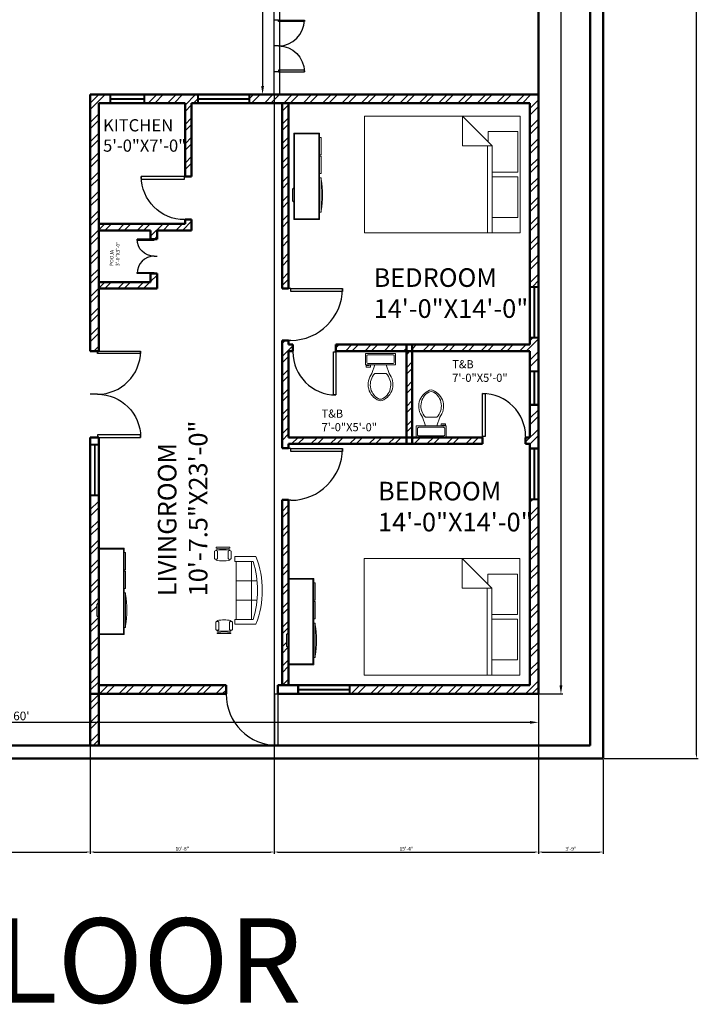
# Model space of a CAD drawing. Units: inches. Extents: x -12550 to 6516, y 1273 to 18700.
# Tile 17 of 19: x 6043 to 6516, y 1273 to 1958. Entities that reach past the tile are written whole.
import ezdxf

# ---------------------------------------------------------------- set-up
doc = ezdxf.new("R2010")
doc.units = ezdxf.units.IN
for name, color, linetype, lineweight in [('A-ANNO-DIMS', 2, 'Continuous', 18), ('A-ANNO-TEXT', 7, 'Continuous', 25), ('A-AREA-IDEN', 1, 'Continuous', 18), ('A-DOOR', 5, 'Continuous', 25), ('A-EQPM', 4, 'Continuous', 25), ('A-FURN', 8, 'Continuous', 18), ('A-GLAZ', 3, 'Continuous', 25), ('A-WALL', 7, 'Continuous', 50), ('A-WALL-PATT', 8, 'Continuous', 13)]:
    doc.layers.add(name, color=color, linetype=linetype, lineweight=lineweight)
doc.styles.get("Standard").update_dxf_attribs({"font": 'arial.ttf'})
doc.dimstyles.new('ISO-25', dxfattribs={"dimtxt": 2.5, "dimasz": 2.5, "dimexe": 1.25, "dimexo": 0.625, "dimtad": 1, "dimlunit": 4, "dimtxsty": 'Standard', "dimcen": 2.5, "dimadec": 0, "dimazin": 0, "dimtfac": 1, "dimtmove": 0, "dimatfit": 3, "dimfxl": 1, "dimarcsym": 0})
pattern_1 = [(45, (3666.851, 0), (-6.735192, 6.735192), []), (45, (3671.341, 0), (-6.735192, 6.735192), [])]

# ---------------------------------------------------------------- blocks, each defined once
blk = doc.blocks.new('*U2')
for p, q in [((0, 0), (0, -5)), ((30, 0), (30, -5))]:
    blk.add_line(p, q)
blk.add_lwpolyline([(0, 0), (0, 30), (1.75, 30), (1.75, 0)], close=True)
blk.add_arc((0, 0), 30, 0, 90)
blk = doc.blocks.new('Bed - Queen')
for p, q in [((0, -80.00003), (0, 0)), ((0, 0), (59.99999, 0)), ((59.99999, 0), (59.99999, -80.00003)), ((7.99999, -1.2), (28.79998, -1.2)), ((7.99999, -14.4), (7.99999, -1.2)), ((28.79998, -1.2), (28.79998, -14.4)), ((31.19999, -1.2), (51.99999, -1.2)), ((31.19999, -14.4), (31.19999, -1.2)), ((51.99999, -1.2), (51.99999, -16.4)), ((0, -14.4), (44.8, -14.4)), ((59.99999, -29.6), (44.8, -14.4)), ((44.8, -14.4), (44.8, -29.6)), ((44.8, -16.8), (0, -16.8)), ((51.99999, -16.4), (46.79936, -16.4)), ((44.8, -29.6), (59.99999, -29.6)), ((59.99999, -80.00003), (0, -80.00003))]:
    blk.add_line(p, q)
blk = doc.blocks.new('Toilet - top')
for p, q in [((9.5, -6), (9.5, -2)), ((-10, -8.5), (-8, -8.5)), ((-10, -9.5), (-10, -8.5)), ((-7, -9.5), (-10, -9.5)), ((-8, -8.5), (-8, -8)), ((-7, -8), (-7, -9.5)), ((-4, -8), (-6, -14)), ((4, -8), (6, -14)), ((4, -14), (-4, -14))]:
    blk.add_line(p, q)
blk.add_lwpolyline([(10.5, -8), (10.5, 0), (-10.5, 0), (-10.5, -8)], close=True)
for points in [[(-9.5, -2), (-9.5, -6)], [(8.5, -1), (-8.5, -1)], [(-8.5, -7), (8.5, -7)]]:
    blk.add_lwpolyline(points)
for centre, radius, start, end in [((-8.62, -1.88), 0.884, 81.8699, 188.1301), ((-8.62, -6.12), 0.884, 171.8699, 278.1301), ((8.62, -1.88), 0.884, 351.8699, 98.1301), ((8.62, -6.12), 0.884, 261.8699, 8.1301), ((3.52, -21.58), 12.17, 141.46911, 247.97143), ((4.2, -21.82), 11.33, 136.36773, 238.94682), ((-3.52, -21.58), 12.17, 292.02843, 38.53071), ((-4.2, -21.82), 11.33, 301.05301, 43.63209), ((0, -27.88), 4, 245.73182, 294.26817), ((0, -29), 4, 254.86053, 285.13947)]:
    blk.add_arc(centre, radius, start, end)
blk = doc.blocks.new('Entertainment Center')
for p, q in [((-4, 0), (-5, -1)), ((4, 0), (-4, 0)), ((5, -1), (4, 0)), ((-17, -19), (-17, -1)), ((-17, -1), (43, -1)), ((-16.5, -18.5), (-16.5, -1.5)), ((-16.5, -1.5), (42.5, -1.5)), ((42.5, -1.5), (42.5, -18.5)), ((43, -1), (43, -19)), ((43, -19), (-17, -19)), ((42.5, -18.5), (-16.5, -18.5)), ((-12, -20), (-12, -19)), ((12, -20), (-12, -20)), ((12, -19), (12, -20)), ((15, -20), (15, -19)), ((27, -20), (15, -20)), ((27, -19), (27, -20)), ((28, -20), (28, -19)), ((40, -20), (28, -20)), ((40, -19), (40, -20))]:
    blk.add_line(p, q)
blk.add_arc((0, 40), 61, 259.6111, 280.3889)
blk = doc.blocks.new('Sofa - Roundback 7 ft.')
for p, q in [((-36.000027, -34), (-36.000027, -11.4696)), ((-12.00002, -32.4421), (-12.00003, -6.5971)), ((11.99997, -32.4421), (11.99998, -6.5971)), ((35.99998, -34), (35.99998, -11.4696)), ((-35.999844, -13.3819), (35.9998, -13.3819)), ((-36.000027, -32.4421), (35.99998, -32.4421))]:
    blk.add_line(p, q)
for points in [[(-36.000027, -34), (-42.000027, -34), (-42.000027, -8)], [(41.99998, -8), (41.99998, -34), (35.99998, -34)]]:
    blk.add_lwpolyline(points)
for centre, radius, start, end in [((0, -114.25), 114.25, 68.43141, 111.5686), ((-0.00001, -127.1968), 121.1968, 72.72033, 107.2797)]:
    blk.add_arc(centre, radius, start, end)
blk = doc.blocks.new('Chair - Desk')
for p, q in [((-8.5, 0), (-8.5, -1)), ((-8.5, 0), (8.5, 0)), ((8.5, 0), (8.5, -1)), ((-10.5, -5), (-10.5, -14)), ((-8.5, -3), (-8.5, -4)), ((-8.5, -3), (8.5, -3)), ((-6.5, -14), (-6.5, -5)), ((-2, -3), (-2, -1.9355)), ((2, -1.9576), (2, -3)), ((6.5, -5), (6.5, -14)), ((8.5, -3), (8.5, -4)), ((10.5, -14), (10.5, -5)), ((-8.5, -15), (-8.5, -16)), ((8.5, -15), (8.5, -16))]:
    blk.add_line(p, q)
for centre, radius, start, end in [((-8.5, -6.5), 2.5, 36.8699, 143.1301), ((0, 34.625), 36.625, 256.5803, 283.4197), ((8.5, -6.5), 2.5, 36.8699, 143.1301), ((-8.5, -12.5), 2.5, 216.8699, 323.1301), ((0, 19.625), 36.625, 256.5803, 283.4197), ((8.5, -12.5), 2.5, 216.8699, 323.1301)]:
    blk.add_arc(centre, radius, start, end)
blk = doc.blocks.new('*D52')
at = {"layer": 'A-ANNO-DIMS', "color": 0, "lineweight": -2, "transparency": 16777216}
for p, q in [((6219.91, 2056.25), (6211.2, 2056.25)), ((6212.45, 2050.25), (6212.45, 1912.25)), ((6219.91, 1906.25), (6211.2, 1906.25))]:
    blk.add_line(p, q, dxfattribs=at)
at = {"layer": 'A-ANNO-DIMS', "color": 0, "transparency": 16777216}
for points in [[(6211.45, 2050.25), (6213.45, 2050.25), (6212.45, 2056.25)], [(6211.45, 1912.25), (6213.45, 1912.25), (6212.45, 1906.25)]]:
    blk.add_solid(points, dxfattribs=at)
at = {"layer": 'Defpoints', "color": 0, "transparency": 16777216}
for p in [(6220.54, 2056.25), (6212.45, 1906.25), (6220.54, 1906.25)]:
    blk.add_point(p, dxfattribs=at)
at = {"layer": 'A-ANNO-DIMS', "color": 0, "transparency": 16777216, "insert": (6208.76, 1981.25), "char_height": 6, "attachment_point": 5, "rotation": 90}
blk.add_mtext('12\'-6"', dxfattribs=at)
blk = doc.blocks.new('*D54')
at = {"layer": 'A-ANNO-DIMS', "color": 0, "lineweight": -2, "transparency": 16777216}
for p, q in [((6405.16, 2473.25), (6421.41, 2473.25)), ((6420.16, 2467.25), (6420.16, 1495.25)), ((6405.16, 1489.25), (6421.41, 1489.25))]:
    blk.add_line(p, q, dxfattribs=at)
at = {"layer": 'A-ANNO-DIMS', "color": 0, "transparency": 16777216}
for points in [[(6419.16, 2467.25), (6421.16, 2467.25), (6420.16, 2473.25)], [(6419.16, 1495.25), (6421.16, 1495.25), (6420.16, 1489.25)]]:
    blk.add_solid(points, dxfattribs=at)
at = {"layer": 'Defpoints', "color": 0, "transparency": 16777216}
for p in [(6404.54, 2473.25), (6404.54, 1489.25), (6420.16, 1489.25)]:
    blk.add_point(p, dxfattribs=at)
at = {"layer": 'A-ANNO-DIMS', "color": 0, "transparency": 16777216, "insert": (6416.47, 1981.25), "char_height": 6, "attachment_point": 5, "rotation": 90}
blk.add_mtext("82'", dxfattribs=at)
blk = doc.blocks.new('*D55')
at = {"layer": 'A-ANNO-DIMS', "color": 0, "lineweight": -2, "transparency": 16777216}
for p, q in [((5684.54, 1488.62), (5684.54, 1468.21)), ((6404.54, 1488.62), (6404.54, 1468.21)), ((6398.54, 1469.46), (5690.54, 1469.46))]:
    blk.add_line(p, q, dxfattribs=at)
at = {"layer": 'A-ANNO-DIMS', "color": 0, "transparency": 16777216}
for points in [[(5690.54, 1470.46), (5690.54, 1468.46), (5684.54, 1469.46)], [(6398.54, 1470.46), (6398.54, 1468.46), (6404.54, 1469.46)]]:
    blk.add_solid(points, dxfattribs=at)
at = {"layer": 'Defpoints', "color": 0, "transparency": 16777216}
for p in [(5684.54, 1489.25), (6404.54, 1489.25), (5684.54, 1469.46)]:
    blk.add_point(p, dxfattribs=at)
at = {"layer": 'A-ANNO-DIMS', "color": 0, "transparency": 16777216, "insert": (6044.54, 1473.15), "char_height": 6, "attachment_point": 5}
blk.add_mtext("60'", dxfattribs=at)
blk = doc.blocks.new('WIN-3FT')
for p, q in [((0, 0), (0, 6)), ((0, 6), (36.02, 6)), ((36.02, 0), (0, 0)), ((0.5, 0), (0.5, 6)), ((35.52, 3.2), (0.5, 3.2)), ((35.52, 2.8), (0.5, 2.8)), ((35.52, 6), (35.52, 0)), ((36.02, 6), (36.02, 0))]:
    blk.add_line(p, q)
blk = doc.blocks.new('WIN-2FT')
for p, q in [((0, 0), (0, 24.02)), ((0, 24.02), (6, 24.02)), ((0, 23.52), (6, 23.52)), ((2.8, 0.5), (2.8, 23.52)), ((3.2, 0.5), (3.2, 23.52)), ((6, 24.02), (6, 0)), ((6, 0.5), (0, 0.5)), ((6, 0), (0, 0))]:
    blk.add_line(p, q)
blk = doc.blocks.new('*D122')
at = {"layer": 'A-ANNO-DIMS', "color": 0, "lineweight": -2, "transparency": 16777216}
for p, q in [((6450.16, 2518.25), (6515.79, 2518.25)), ((6514.54, 1446.75), (6514.54, 2515.75)), ((6450.16, 1444.25), (6515.79, 1444.25))]:
    blk.add_line(p, q, dxfattribs=at)
at = {"layer": 'A-ANNO-DIMS', "color": 0, "transparency": 16777216}
for points in [[(6514.12, 2515.75), (6514.96, 2515.75), (6514.54, 2518.25)], [(6514.12, 1446.75), (6514.96, 1446.75), (6514.54, 1444.25)]]:
    blk.add_solid(points, dxfattribs=at)
at = {"layer": 'Defpoints', "color": 0, "transparency": 16777216}
for p in [(6449.54, 2518.25), (6514.54, 2518.25), (6449.54, 1444.25)]:
    blk.add_point(p, dxfattribs=at)
at = {"layer": 'A-ANNO-DIMS', "color": 0, "transparency": 16777216, "insert": (6512.64, 1981.25), "char_height": 2.5, "attachment_point": 5, "rotation": 90}
blk.add_mtext('89\'-6"', dxfattribs=at)
blk = doc.blocks.new('*D124')
at = {"layer": 'A-ANNO-DIMS', "color": 0, "lineweight": -2, "transparency": 16777216}
for p, q in [((5684.54, 1488.62), (5684.54, 1378)), ((6092.54, 1488.62), (6092.54, 1378)), ((5687.04, 1379.25), (6090.04, 1379.25))]:
    blk.add_line(p, q, dxfattribs=at)
at = {"layer": 'A-ANNO-DIMS', "color": 0, "transparency": 16777216}
for points in [[(5687.04, 1379.66), (5687.04, 1378.83), (5684.54, 1379.25)], [(6090.04, 1379.66), (6090.04, 1378.83), (6092.54, 1379.25)]]:
    blk.add_solid(points, dxfattribs=at)
at = {"layer": 'Defpoints', "color": 0, "transparency": 16777216}
for p in [(5684.54, 1489.25), (6092.54, 1489.25), (6092.54, 1379.25)]:
    blk.add_point(p, dxfattribs=at)
at = {"layer": 'A-ANNO-DIMS', "color": 0, "transparency": 16777216, "insert": (5888.54, 1381.15), "char_height": 2.5, "attachment_point": 5}
blk.add_mtext('34\'-0"', dxfattribs=at)
blk = doc.blocks.new('*D125')
at = {"layer": 'A-ANNO-DIMS', "color": 0, "lineweight": -2, "transparency": 16777216}
for p, q in [((6220.54, 1905.62), (6220.54, 1378)), ((6092.54, 1488.62), (6092.54, 1378)), ((6095.04, 1379.25), (6218.04, 1379.25))]:
    blk.add_line(p, q, dxfattribs=at)
at = {"layer": 'A-ANNO-DIMS', "color": 0, "transparency": 16777216}
for points in [[(6095.04, 1379.66), (6095.04, 1378.83), (6092.54, 1379.25)], [(6218.04, 1379.66), (6218.04, 1378.83), (6220.54, 1379.25)]]:
    blk.add_solid(points, dxfattribs=at)
at = {"layer": 'Defpoints', "color": 0, "transparency": 16777216}
for p in [(6220.54, 1906.25), (6092.54, 1489.25), (6220.54, 1379.25)]:
    blk.add_point(p, dxfattribs=at)
at = {"layer": 'A-ANNO-DIMS', "color": 0, "transparency": 16777216, "insert": (6156.54, 1381.15), "char_height": 2.5, "attachment_point": 5}
blk.add_mtext('10\'-8"', dxfattribs=at)
blk = doc.blocks.new('*D126')
at = {"layer": 'A-ANNO-DIMS', "color": 0, "lineweight": -2, "transparency": 16777216}
for p, q in [((6220.54, 1905.62), (6220.54, 1378)), ((6404.54, 1905.62), (6404.54, 1378)), ((6223.04, 1379.25), (6402.04, 1379.25))]:
    blk.add_line(p, q, dxfattribs=at)
at = {"layer": 'A-ANNO-DIMS', "color": 0, "transparency": 16777216}
for points in [[(6223.04, 1379.66), (6223.04, 1378.83), (6220.54, 1379.25)], [(6402.04, 1379.66), (6402.04, 1378.83), (6404.54, 1379.25)]]:
    blk.add_solid(points, dxfattribs=at)
at = {"layer": 'Defpoints', "color": 0, "transparency": 16777216}
for p in [(6220.54, 1906.25), (6404.54, 1906.25), (6404.54, 1379.25)]:
    blk.add_point(p, dxfattribs=at)
at = {"layer": 'A-ANNO-DIMS', "color": 0, "transparency": 16777216, "insert": (6312.54, 1381.15), "char_height": 2.5, "attachment_point": 5}
blk.add_mtext('15\'-4"', dxfattribs=at)
blk = doc.blocks.new('*D127')
at = {"layer": 'A-ANNO-DIMS', "color": 0, "lineweight": -2, "transparency": 16777216}
for p, q in [((6404.54, 1488.62), (6404.54, 1378)), ((6449.54, 1443.62), (6449.54, 1378)), ((6407.04, 1379.25), (6447.04, 1379.25))]:
    blk.add_line(p, q, dxfattribs=at)
at = {"layer": 'A-ANNO-DIMS', "color": 0, "transparency": 16777216}
for points in [[(6407.04, 1379.66), (6407.04, 1378.83), (6404.54, 1379.25)], [(6447.04, 1379.66), (6447.04, 1378.83), (6449.54, 1379.25)]]:
    blk.add_solid(points, dxfattribs=at)
at = {"layer": 'Defpoints', "color": 0, "transparency": 16777216}
for p in [(6404.54, 1489.25), (6449.54, 1444.25), (6449.54, 1379.25)]:
    blk.add_point(p, dxfattribs=at)
at = {"layer": 'A-ANNO-DIMS', "color": 0, "transparency": 16777216, "insert": (6427.04, 1381.15), "char_height": 2.5, "attachment_point": 5}
blk.add_mtext('3\'-9"', dxfattribs=at)

msp = doc.modelspace()

# ---------------------------------------------------------------- hatches: boundary and pattern name
at = {"layer": 'A-WALL-PATT'}
h = msp.add_hatch(dxfattribs=at)
h.set_pattern_fill('ANSI32', color=256)
h.set_pattern_definition(pattern_1)
h.paths.add_polyline_path([(6106.297, 1906.247), (6092.54, 1906.247), (6092.54, 1727.747), (6097.54, 1727.747), (6098.54, 1727.747), (6098.54, 1900.247), (6106.297, 1900.247)])
h = msp.add_hatch(dxfattribs=at)
h.set_pattern_fill('ANSI32', color=256)
h.set_pattern_definition(pattern_1)
h.paths.add_polyline_path([(6167.378, 1906.247), (6130.314, 1906.247), (6130.314, 1900.247), (6158.54, 1900.247), (6158.54, 1849.247), (6163.04, 1849.247), (6163.04, 1900.247), (6167.378, 1900.247)])
h = msp.add_hatch(dxfattribs=at)
h.set_pattern_fill('ANSI32', color=256)
h.set_pattern_definition(pattern_1)
h.paths.add_polyline_path([(6404.54, 1906.247), (6226.04, 1906.247), (6203.396, 1906.247), (6203.396, 1900.247), (6226.04, 1900.247), (6398.54, 1900.247), (6398.54, 1772.747), (6404.54, 1772.747)])
h = msp.add_hatch(dxfattribs=at)
h.set_pattern_fill('ANSI32', color=256)
h.set_pattern_definition(pattern_1)
h.paths.add_polyline_path([(6230.54, 1900.247), (6226.04, 1900.247), (6226.04, 1771.247), (6230.54, 1771.247)])
h = msp.add_hatch(dxfattribs=at)
h.set_pattern_fill('ANSI32', color=256)
h.set_pattern_definition(pattern_1)
h.paths.add_polyline_path([(6163.04, 1819.247), (6158.54, 1819.247), (6158.54, 1816.247), (6098.54, 1816.247), (6098.54, 1811.747), (6134.54, 1811.747), (6134.54, 1805.747), (6137.04, 1805.747), (6139.04, 1805.747), (6139.04, 1811.747), (6163.04, 1811.747)])
h = msp.add_hatch(dxfattribs=at)
h.set_pattern_fill('ANSI32', color=256)
h.set_pattern_definition(pattern_1)
h.paths.add_polyline_path([(6139.04, 1781.747), (6137.04, 1781.747), (6134.54, 1781.747), (6134.54, 1775.747), (6098.54, 1775.747), (6098.54, 1771.247), (6139.04, 1771.247)])
h = msp.add_hatch(dxfattribs=at)
h.set_pattern_fill('ANSI32', color=256)
h.set_pattern_definition(pattern_1)
h.paths.add_polyline_path([(6230.54, 1727.747), (6233.54, 1727.747), (6233.54, 1732.247), (6230.54, 1732.247), (6230.54, 1735.247), (6226.04, 1735.247), (6226.04, 1660.247), (6230.54, 1660.247), (6230.54, 1663.247), (6233.492, 1663.247), (6312.54, 1663.247), (6312.54, 1667.747), (6233.492, 1667.747), (6230.54, 1667.747)])
h = msp.add_hatch(dxfattribs=at)
h.set_pattern_fill('ANSI32', color=256)
h.set_pattern_definition(pattern_1)
h.paths.add_polyline_path([(6404.54, 1736.73), (6398.54, 1736.73), (6398.54, 1732.247), (6395.54, 1732.247), (6316.54, 1732.247), (6316.54, 1727.747), (6395.54, 1727.747), (6398.54, 1727.747), (6398.54, 1714.042), (6404.54, 1714.042)])
h = msp.add_hatch(dxfattribs=at)
h.set_pattern_fill('ANSI32', color=256)
h.set_pattern_definition(pattern_1)
h.paths.add_polyline_path([(6312.54, 1732.247), (6263.54, 1732.247), (6263.54, 1727.747), (6312.54, 1727.747)], flags=17)
h = msp.add_hatch(dxfattribs=at)
h.set_pattern_fill('ANSI32', color=256)
h.set_pattern_definition(pattern_1)
h.paths.add_polyline_path([(6316.54, 1727.747), (6312.54, 1727.747), (6312.54, 1667.747), (6316.54, 1667.747)])
h = msp.add_hatch(dxfattribs=at)
h.set_pattern_fill('ANSI32', color=256)
h.set_pattern_definition(pattern_1)
h.paths.add_polyline_path([(6404.54, 1690.024), (6398.54, 1690.024), (6398.54, 1667.747), (6395.54, 1667.747), (6395.54, 1663.247), (6398.54, 1663.247), (6398.54, 1660.369), (6404.54, 1660.369)])
h = msp.add_hatch(dxfattribs=at)
h.set_pattern_fill('ANSI32', color=256)
h.set_pattern_definition(pattern_1)
h.paths.add_polyline_path([(6365.54, 1667.747), (6316.54, 1667.747), (6316.54, 1663.247), (6365.54, 1663.247)])
h = msp.add_hatch(dxfattribs=at)
h.set_pattern_fill('ANSI32', color=256)
h.set_pattern_definition(pattern_1)
h.paths.add_polyline_path([(6187.04, 1495.247), (6098.54, 1495.247), (6098.54, 1530.559), (6098.04, 1530.559), (6098.04, 1542.559), (6097.04, 1543.559), (6097.04, 1551.559), (6098.04, 1552.559), (6098.04, 1590.559), (6098.276, 1627.032), (6092.54, 1627.032), (6092.54, 1489.247), (6187.04, 1489.247)])
h = msp.add_hatch(dxfattribs=at)
h.set_pattern_fill('ANSI32', color=256)
h.set_pattern_definition(pattern_1)
h.paths.add_polyline_path([(6226.04, 1623.947), (6226.04, 1495.247), (6230.54, 1495.247), (6230.54, 1509.575), (6230.04, 1509.575), (6230.04, 1521.575), (6229.04, 1522.575), (6229.04, 1530.575), (6230.04, 1531.575), (6230.04, 1569.575), (6230.537, 1623.947)])
h = msp.add_hatch(dxfattribs=at)
h.set_pattern_fill('ANSI32', color=256)
h.set_pattern_definition(pattern_1)
h.paths.add_polyline_path([(6404.54, 1624.352), (6398.54, 1624.352), (6398.54, 1495.247), (6273.126, 1495.247), (6273.126, 1489.247), (6404.54, 1489.247)])
h = msp.add_hatch(dxfattribs=at)
h.set_pattern_fill('ANSI32', color=256)
h.set_pattern_definition(pattern_1)
h.paths.add_polyline_path([(6098.54, 1489.247), (6092.54, 1489.247), (6092.54, 1453.247), (6098.54, 1453.247)])

# ---------------------------------------------------------------- linework, layer by layer
at = {"layer": 'A-EQPM'}
for p, q in [((6220.54, 1906.247), (6220.54, 2056.247)), ((6224.54, 1906.247), (6224.54, 2056.247)), ((6404.54, 2056.247), (6404.54, 1906.247)), ((6404.54, 1906.247), (6220.54, 1906.247))]:
    msp.add_line(p, q, dxfattribs=at)
at = {"layer": 'A-WALL'}
for p, q in [((6449.54, 2518.247), (6449.54, 1444.247)), ((6440.54, 2509.247), (6440.54, 1453.247)), ((6404.54, 1489.247), (6404.54, 2060.923)), ((6440.54, 1489.247), (6440.54, 2060.923)), ((6226.04, 1906.247), (6092.54, 1906.247)), ((6092.54, 1727.747), (6092.54, 1906.247)), ((6404.54, 1906.247), (6226.04, 1906.247)), ((6158.54, 1900.247), (6098.54, 1900.247)), ((6098.54, 1727.747), (6098.54, 1900.247)), ((6158.54, 1849.247), (6158.54, 1900.247)), ((6226.04, 1900.247), (6163.04, 1900.247)), ((6163.04, 1849.247), (6163.04, 1900.247)), ((6398.54, 1900.247), (6226.04, 1900.247)), ((6226.04, 1771.247), (6226.04, 1900.247)), ((6230.54, 1771.247), (6230.54, 1900.247)), ((6398.54, 1732.247), (6398.54, 1900.247)), ((6158.54, 1849.247), (6163.04, 1849.247)), ((6158.54, 1816.247), (6098.54, 1816.247)), ((6158.54, 1816.247), (6158.54, 1819.247)), ((6163.04, 1819.247), (6158.54, 1819.247)), ((6163.04, 1811.747), (6163.04, 1819.247)), ((6163.04, 1816.247), (6163.04, 1819.247)), ((6134.54, 1811.747), (6098.54, 1811.747)), ((6134.54, 1805.747), (6134.54, 1811.747)), ((6163.04, 1811.747), (6139.04, 1811.747)), ((6139.04, 1805.747), (6139.04, 1811.747)), ((6134.54, 1805.747), (6139.04, 1805.747)), ((6134.54, 1775.747), (6134.54, 1781.747)), ((6139.04, 1781.747), (6134.54, 1781.747)), ((6139.04, 1771.247), (6139.04, 1781.747)), ((6139.04, 1775.747), (6139.04, 1781.747)), ((6134.54, 1775.747), (6098.54, 1775.747)), ((6139.04, 1771.247), (6098.54, 1771.247)), ((6226.04, 1771.247), (6230.54, 1771.247)), ((6226.04, 1660.247), (6226.04, 1735.247)), ((6230.54, 1735.247), (6226.04, 1735.247)), ((6230.54, 1732.247), (6230.54, 1735.247)), ((6230.54, 1732.247), (6230.54, 1735.247)), ((6230.54, 1732.247), (6230.54, 1735.247)), ((6230.54, 1732.247), (6230.54, 1735.247)), ((6098.54, 1727.747), (6092.54, 1727.747)), ((6233.54, 1732.247), (6230.54, 1732.247)), ((6233.54, 1727.747), (6230.54, 1727.747)), ((6230.54, 1667.747), (6230.54, 1727.747)), ((6230.54, 1667.747), (6230.54, 1727.747)), ((6230.54, 1667.747), (6230.54, 1727.747)), ((6230.54, 1727.747), (6233.54, 1727.747)), ((6233.54, 1727.747), (6233.54, 1732.247)), ((6395.54, 1732.247), (6263.54, 1732.247)), ((6263.54, 1732.247), (6263.54, 1727.747)), ((6395.54, 1727.747), (6263.54, 1727.747)), ((6312.54, 1663.247), (6312.54, 1732.247)), ((6316.54, 1663.247), (6316.54, 1732.247)), ((6398.54, 1732.247), (6395.54, 1732.247)), ((6398.54, 1732.247), (6395.54, 1732.247)), ((6398.54, 1727.747), (6395.54, 1727.747)), ((6398.54, 1667.747), (6398.54, 1727.747)), ((6098.54, 1667.747), (6092.54, 1667.747)), ((6092.54, 1453.247), (6092.54, 1667.747)), ((6098.54, 1453.247), (6098.54, 1667.747)), ((6233.492, 1667.747), (6230.54, 1667.747)), ((6365.54, 1667.747), (6233.492, 1667.747)), ((6365.54, 1667.747), (6365.54, 1663.247)), ((6398.54, 1667.747), (6395.54, 1667.747)), ((6395.54, 1663.247), (6395.54, 1667.747)), ((6226.04, 1663.247), (6226.04, 1660.247)), ((6226.04, 1660.247), (6230.54, 1660.247)), ((6233.492, 1663.247), (6230.54, 1663.247)), ((6230.54, 1660.247), (6230.54, 1663.247)), ((6230.54, 1660.247), (6230.54, 1663.247)), ((6230.54, 1660.247), (6230.54, 1663.247)), ((6365.54, 1663.247), (6233.492, 1663.247)), ((6398.54, 1663.247), (6395.54, 1663.247)), ((6398.54, 1663.247), (6395.54, 1663.247)), ((6398.54, 1495.247), (6398.54, 1663.247)), ((6226.04, 1495.247), (6226.04, 1624.247)), ((6230.54, 1624.247), (6226.04, 1624.247)), ((6230.54, 1495.247), (6230.54, 1624.247)), ((6187.04, 1495.247), (6098.54, 1495.247)), ((6187.04, 1489.247), (6187.04, 1495.247)), ((6398.54, 1495.247), (6223.04, 1495.247)), ((6226.04, 1495.247), (6223.04, 1495.247)), ((6223.04, 1495.247), (6223.04, 1489.247)), ((6187.04, 1489.247), (6092.54, 1489.247)), ((6404.54, 1489.247), (6223.04, 1489.247)), ((5648.54, 1453.247), (6440.54, 1453.247)), ((6187.04, 1453.247), (5923.04, 1453.247)), ((5639.54, 1444.247), (6449.54, 1444.247))]:
    msp.add_line(p, q, dxfattribs=at)

# ---------------------------------------------------------------- block references
at = {"layer": 'A-DOOR', "xscale": -1}
for p, rotation in [((6158.04, 1849.247), 90), ((6097.54, 1667.747), 270)]:
    msp.add_blockref('*U2', p, dxfattribs=dict(at, rotation=rotation))
at = {"layer": 'A-DOOR'}
for p, xscale, yscale, zscale, rotation in [((6137.04, 1805.747), -0.399999999999997, 0.399999999999997, 0.399999999999997, 90), ((6137.04, 1781.747), 0.399999999999997, 0.399999999999997, 0.399999999999997, 90.00000000000003), ((6232.04, 1771.247), 1.199999999999999, 1.199999999999999, 1.199999999999999, 270), ((6232.04, 1659.947), 1.199999999999999, 1.199999999999999, 1.199999999999999, 270), ((6223.04, 1489.247), 1.199999999999999, 1.199999999999999, 1.199999999999999, 180)]:
    msp.add_blockref('*U2', p, dxfattribs=dict(at, xscale=xscale, yscale=yscale, zscale=zscale, rotation=rotation))
for p, rotation in [((6097.54, 1727.747), 270), ((6263.54, 1727.247), 180)]:
    msp.add_blockref('*U2', p, dxfattribs=dict(at, rotation=rotation))
msp.add_blockref('*U2', (6365.54, 1668.247), dxfattribs=at)
at = {"layer": 'A-EQPM', "yscale": 0.5999999999999954, "zscale": 0.5999999999999954, "rotation": 270}
for p, xscale in [((6223.54, 1958.135), 0.5999999999999954), ((6223.54, 1922.135), -0.5999999999999954)]:
    msp.add_blockref('*U2', p, dxfattribs=dict(at, xscale=xscale))
at = {"layer": 'A-FURN'}
for name, p, xscale, yscale, zscale, rotation in [('Bed - Queen', (6391.719, 1809.994), -1.354827908062564, 1.354827908062564, 1.354827908062564, 270), ('Sofa - Roundback 7 ft.', (6212.259, 1561.265), 0.5595223685495907, 0.5595223685495907, 0.5595223685495907, 270), ('Bed - Queen', (6391.559, 1502.217), -1.354827908062564, 1.354827908062564, 1.354827908062564, 270), ('Chair - Desk', (6185.673, 1531.281), 0.5595223685495907, 0.5595223685495907, 0.5595223685495907, 180)]:
    msp.add_blockref(name, p, dxfattribs=dict(at, xscale=xscale, yscale=yscale, zscale=zscale, rotation=rotation))
for name, p, rotation in [('Entertainment Center', (6233.169, 1836.379), 89.99999999999999), ('Toilet - top', (6329.808, 1667.747), 180), ('Entertainment Center', (6097.04, 1547.559), 89.99999999999999), ('Entertainment Center', (6229.04, 1526.575), 89.99999999999999)]:
    msp.add_blockref(name, p, dxfattribs=dict(at, rotation=rotation))
msp.add_blockref('Toilet - top', (6294.562, 1726.198), dxfattribs=at)
at = {"layer": 'A-FURN', "xscale": 0.5595223685495907, "yscale": 0.5595223685495907, "zscale": 0.5595223685495907}
msp.add_blockref('Chair - Desk', (6184.819, 1591.265), dxfattribs=at)
at = {"layer": 'A-GLAZ'}
for name, p, rotation in [('WIN-2FT', (6106.296, 1906.247), 269.9999999999974), ('WIN-3FT', (6203.395, 1906.247), 180), ('WIN-3FT', (6404.54, 1736.73), 89.99999999999638), ('WIN-2FT', (6404.539, 1714.042), 180), ('WIN-3FT', (6098.54, 1627.032), 90.0000000000048), ('WIN-3FT', (6404.54, 1624.352), 89.99999999999625), ('WIN-3FT', (6273.125, 1495.247), 180)]:
    msp.add_blockref(name, p, dxfattribs=dict(at, rotation=rotation))

# ---------------------------------------------------------------- texts
at = {"layer": 'A-ANNO-TEXT', "insert": (5840.46, 1333.138), "char_height": 58.816, "attachment_point": 1}
msp.add_mtext('4th FLOOR', dxfattribs=at)
at = {"layer": 'A-AREA-IDEN', "attachment_point": 1}
for s, width, gutter_width, insert, char_height in [('KITCHEN\\P5\'-0"X7\'-0"', 1.29487, 42.422, (6101.42, 1889.124), 8.48435), ('T&B\\P7\'-0"X5\'-0"', 4.19569, 28.328, (6344.462, 1721.465), 5.66556), ('T&B\\P7\'-0"X5\'-0"', 4.19569, 28.328, (6253.552, 1687.107), 5.66556)]:
    msp.add_mtext_dynamic_manual_height_columns(s, width=width, gutter_width=gutter_width, heights=[0], dxfattribs=dict(at, insert=insert, char_height=char_height))
at = {"layer": 'A-AREA-IDEN', "insert": (6106.092, 1787.026), "char_height": 2.5, "attachment_point": 1, "rotation": 89.183853}
msp.add_mtext_dynamic_manual_height_columns('POOJA\\P3\'-0"X3\'-0"', width=0.78585, gutter_width=12.5, heights=[0], dxfattribs=at)
at = {"layer": 'A-AREA-IDEN', "char_height": 12.93169, "attachment_point": 1}
for insert in [(6289.755, 1785.378), (6292.82, 1636.812)]:
    msp.add_mtext('BEDROOM\\P14\'-0"X14\'-0"', dxfattribs=dict(at, insert=insert))
at = {"layer": 'A-AREA-IDEN', "insert": (6139.563, 1557.153), "char_height": 12.93169, "attachment_point": 1, "rotation": 90}
msp.add_mtext('LIVINGROOM\\P10\'-7.5"X23\'-0"', dxfattribs=at)

# ---------------------------------------------------------------- dimensions: what is measured, and where the dimension line sits
at = {"layer": 'A-ANNO-DIMS'}
for base, p1, p2, override, picture, middle in [((6514.54, 2518.247), (6449.54, 1444.247), (6449.54, 2518.247), {"dimdec": 1, "dimlfac": 1, "dimrnd": 0, "dimzin": 1, "dimdsep": 46, "dimlunit": 4, "dimfrac": 2}, '*D122', (6512.638, 1981.247)), ((6420.159, 1489.247), (6404.54, 2473.247), (6404.54, 1489.247), {"dimtxt": 6, "dimasz": 6, "dimclrd": 0, "dimclre": 0, "dimclrt": 0}, '*D54', (6416.471, 1981.247)), ((6212.453, 1906.247), (6220.54, 2056.247), (6220.54, 1906.247), {"dimtxt": 6, "dimasz": 6, "dimclrd": 0, "dimclre": 0, "dimclrt": 0}, '*D52', (6208.764, 1981.247))]:
    dim = msp.add_linear_dim(base=base, p1=p1, p2=p2, angle=90, dimstyle='ISO-25', override=override, dxfattribs=at)
    dim.commit()
    dim.dimension.update_dxf_attribs({"geometry": picture, "text_midpoint": middle})
for base, p1, p2, override, picture, middle in [((6220.54, 1379.247), (6092.54, 1489.247), (6220.54, 1906.247), {"dimdec": 1, "dimlfac": 1, "dimrnd": 0, "dimzin": 1, "dimdsep": 46, "dimlunit": 4, "dimfrac": 2}, '*D125', (6156.54, 1381.149)), ((6404.54, 1379.247), (6220.54, 1906.247), (6404.54, 1906.247), {"dimdec": 1, "dimlfac": 1, "dimrnd": 0, "dimzin": 1, "dimdsep": 46, "dimlunit": 4, "dimfrac": 2}, '*D126', (6312.54, 1381.149)), ((5684.54, 1469.461), (6404.54, 1489.247), (5684.54, 1489.247), {"dimtxt": 6, "dimasz": 6, "dimclrd": 0, "dimclre": 0, "dimclrt": 0}, '*D55', (6044.54, 1473.15)), ((6092.54, 1379.247), (5684.54, 1489.247), (6092.54, 1489.247), {"dimdec": 1, "dimlfac": 1, "dimrnd": 0, "dimzin": 1, "dimdsep": 46, "dimlunit": 4, "dimfrac": 2}, '*D124', (5888.54, 1381.15)), ((6449.54, 1379.247), (6404.54, 1489.247), (6449.54, 1444.247), {"dimdec": 1, "dimlfac": 1, "dimrnd": 0, "dimzin": 1, "dimdsep": 46, "dimlunit": 4, "dimfrac": 2}, '*D127', (6427.04, 1381.15))]:
    dim = msp.add_linear_dim(base=base, p1=p1, p2=p2, dimstyle='ISO-25', override=override, dxfattribs=at)
    dim.commit()
    dim.dimension.update_dxf_attribs({"geometry": picture, "text_midpoint": middle})

doc.saveas('drawing.dxf')
